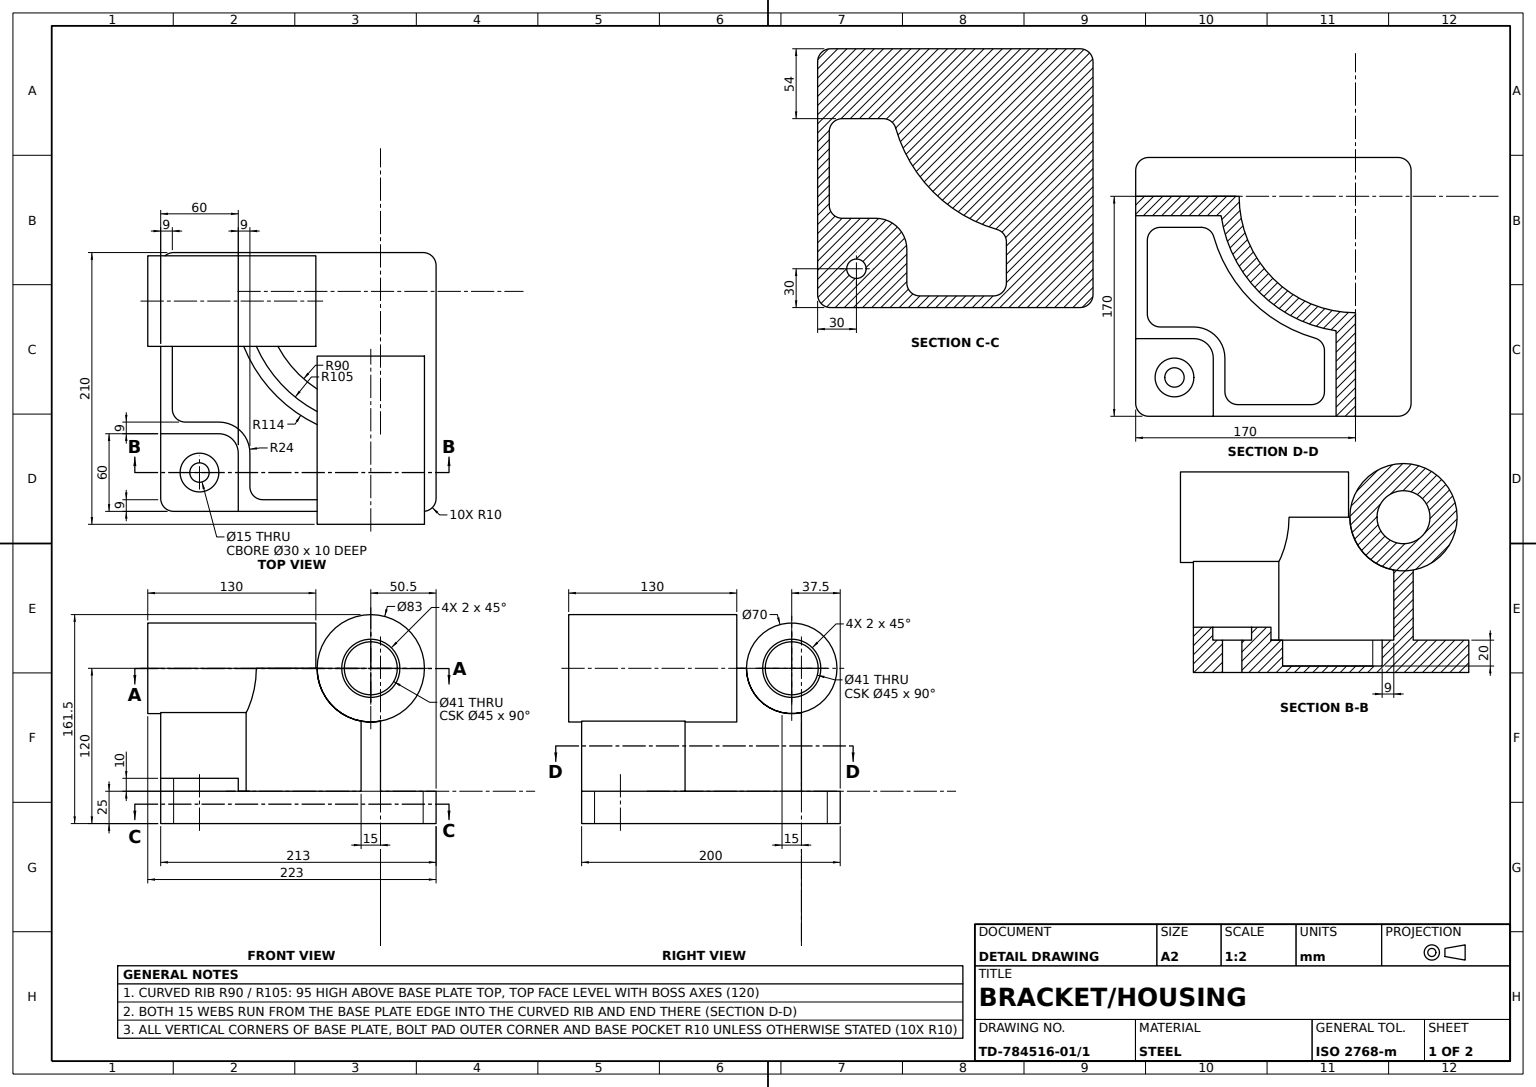
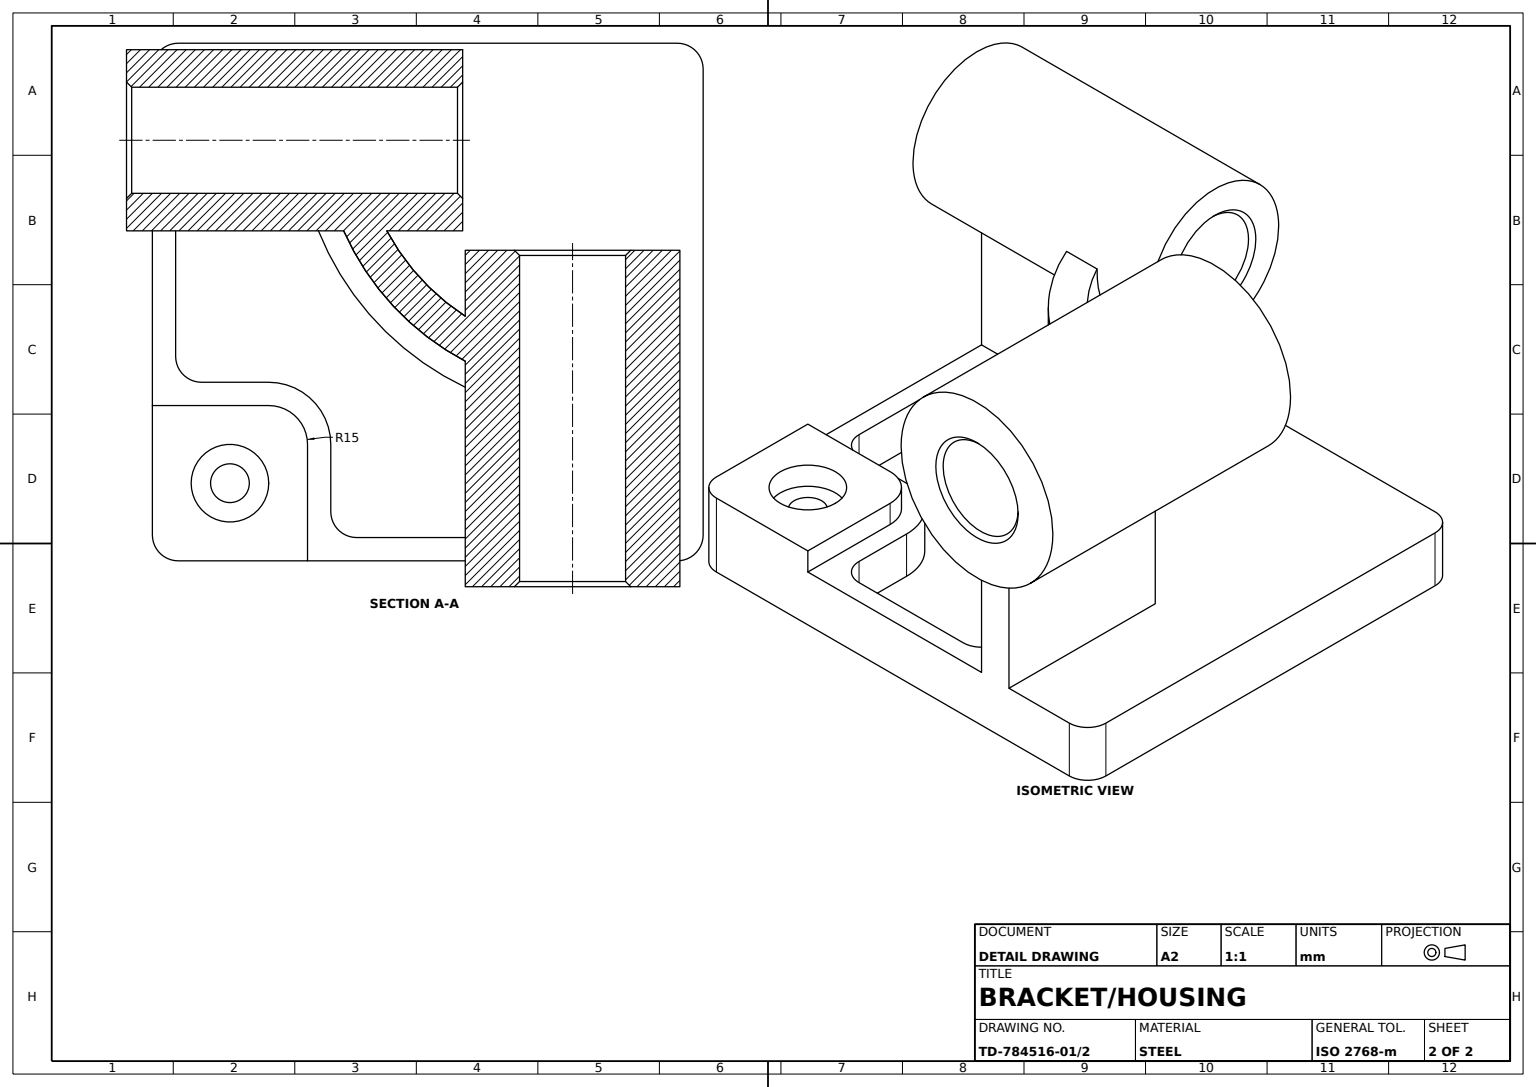
from build123d import *

# Parameters (mm, degrees)
BASE_PLATE_SKETCH_W                       = 200
BASE_PLATE_SKETCH_H                       = 213
BASE_PLATE_DEPTH                          = 25
BOLT_PAD_DEPTH                            = 10
BASE_PLATE_FILLETS_R10_R                  = 10
CENTRAL_HOUSING_DEPTH                     = 95
BEARING_BOSS_A_DEPTH                      = 10
BEARING_BOSS_A_DEPTH_BACK                 = 120
BEARING_BOSS_A_SKETCH_R                   = 35
BEARING_BOSS_B_DEPTH                      = 10
BEARING_BOSS_B_DEPTH_BACK                 = 120
BEARING_BOSS_B_SKETCH_R                   = 41.5
BEARING_BORE_A_41_REACH                   = 298.498
BEARING_BORE_A_SKETCH_R                   = 20.5
BEARING_BORE_B_41_REACH                   = 291.404
BEARING_BORE_B_SKETCH_R                   = 20.5
BORE_CHAMFERS_2X45_SIZE                   = 2
M8_COUNTERBORED_MOUNTING_HOLE_D           = 15
M8_COUNTERBORED_MOUNTING_HOLE_CBORE_D     = 30
M8_COUNTERBORED_MOUNTING_HOLE_CBORE_DEPTH = 10
BASE_POCKET_DEPTH                         = 20


with BuildPart() as part:
    # Base Plate Sketch → Base Plate (new body)
    with BuildSketch(Plane(origin=(0, 0, 0), x_dir=(1, 0, 0), z_dir=(0, 1, 0))):
        Rectangle(BASE_PLATE_SKETCH_W, BASE_PLATE_SKETCH_H)
    extrude(amount=BASE_PLATE_DEPTH)

    # Bolt Pad Sketch → Bolt Pad (add)
    with BuildSketch(Plane(origin=(0, 25, 0), x_dir=(1, 0, 0), z_dir=(0, 1, 0))):
        with BuildLine():
            Line((100, -106.5), (40, -106.5))
            Line((40, -106.5), (40, -61.5))
            ThreePointArc((40, -61.5), (44.393398282, -50.893398282), (55, -46.5))
            Line((55, -46.5), (100, -46.5))
            Line((100, -46.5), (100, -106.5))
        make_face()
    extrude(amount=BOLT_PAD_DEPTH)

    # Base Plate Fillets R10
    base_plate_fillets_r10_edges = [part.edges().sort_by_distance(p)[0] for p in [
        (100, 17.5, 106.5),
        (-100, 12.5, 106.5),
        (-100, 12.5, -106.5),
        (100, 12.5, -106.5),
    ]]
    fillet(base_plate_fillets_r10_edges, radius=BASE_PLATE_FILLETS_R10_R)

    # Central Housing Sketch → Central Housing (add)
    with BuildSketch(Plane(origin=(0, 25, 0), x_dir=(1, 0, 0), z_dir=(0, 1, 0))):
        with BuildLine():
            Line((100, 63.5), (20, 63.5))
            ThreePointArc((20, 63.5), (-6.360389693, -0.139610307), (-70, -26.5))
            Line((-70, -26.5), (-70, -106.5))
            Line((-70, -106.5), (-55, -106.5))
            Line((-55, -106.5), (-55, -40.423048454))
            ThreePointArc((-55, -40.423048454), (4.246212025, -10.746212025), (33.923048454, 48.5))
            Line((33.923048454, 48.5), (100, 48.5))
            Line((100, 48.5), (100, 63.5))
        make_face()
    extrude(amount=CENTRAL_HOUSING_DEPTH)

    # Bearing Boss A Sketch → Bearing Boss A (add, two sides: drawn at the far end of the back side and taken through both)
    with BuildSketch(Plane.XY.offset(106.5).offset(-BEARING_BOSS_A_DEPTH_BACK)):
        with Locations((-62.5, 120)):
            Circle(BEARING_BOSS_A_SKETCH_R)
    extrude(amount=BEARING_BOSS_A_DEPTH + BEARING_BOSS_A_DEPTH_BACK)

    # Bearing Boss B Sketch → Bearing Boss B (add, two sides: drawn at the far end of the back side and taken through both)
    with BuildSketch(Plane(origin=(100, 0, 0), x_dir=(0, 0, -1), z_dir=(1, 0, 0)).offset(-BEARING_BOSS_B_DEPTH_BACK)):
        with Locations((56, 120)):
            Circle(BEARING_BOSS_B_SKETCH_R)
    extrude(amount=BEARING_BOSS_B_DEPTH + BEARING_BOSS_B_DEPTH_BACK)

    # Bearing Bore A Sketch → Bearing Bore A Ø41 (cut, up to next)
    with BuildSketch(Plane.XY.offset(116.5), mode=Mode.PRIVATE) as bearing_bore_a_41_sk1:
        with Locations((-62.5, 120)):
            Circle(BEARING_BORE_A_SKETCH_R)
    bearing_bore_a_41_tool1 = extrude(bearing_bore_a_41_sk1.sketch, amount=-BEARING_BORE_A_41_REACH, mode=Mode.PRIVATE) & part.part
    add(bearing_bore_a_41_tool1.solids().sort_by_distance((-62.5, 120, 116.5))[0], mode=Mode.SUBTRACT)

    # Bearing Bore B Sketch → Bearing Bore B Ø41 (cut, up to next)
    with BuildSketch(Plane(origin=(110, 0, 0), x_dir=(0, 0, -1), z_dir=(1, 0, 0)), mode=Mode.PRIVATE) as bearing_bore_b_41_sk1:
        with Locations((56, 120)):
            Circle(BEARING_BORE_B_SKETCH_R)
    bearing_bore_b_41_tool1 = extrude(bearing_bore_b_41_sk1.sketch, amount=-BEARING_BORE_B_41_REACH, mode=Mode.PRIVATE) & part.part
    add(bearing_bore_b_41_tool1.solids().sort_by_distance((110, 120, -56))[0], mode=Mode.SUBTRACT)

    # Bore Chamfers 2x45°
    bore_chamfers_2x45_edges = [part.edges().sort_by_distance(p)[0] for p in [
        (-83, 120, 116.5),
        (-83, 120, -13.5),
        (110, 120, -35.5),
        (-20, 120, -35.5),
    ]]
    chamfer(bore_chamfers_2x45_edges, length=BORE_CHAMFERS_2X45_SIZE)

    # M8 Counterbored Mounting Hole (through all)
    with Locations(Plane(origin=(70, 35, 76.5), x_dir=(0, 0, 1), z_dir=(0, 1, 0))):
        with Locations((0, 0)):
            CounterBoreHole(M8_COUNTERBORED_MOUNTING_HOLE_D / 2, M8_COUNTERBORED_MOUNTING_HOLE_CBORE_D / 2, M8_COUNTERBORED_MOUNTING_HOLE_CBORE_DEPTH)

    # Base Pocket Sketch → Base Pocket (cut)
    with BuildSketch(Plane(origin=(0, 25, 0), x_dir=(1, 0, 0), z_dir=(0, 1, 0))):
        with BuildLine():
            Line((-46, -55.747641486), (-46, -87.5))
            ThreePointArc((-46, -87.5), (-43.071067812, -94.571067812), (-36, -97.5))
            Line((-36, -97.5), (21, -97.5))
            ThreePointArc((21, -97.5), (28.071067812, -94.571067812), (31, -87.5))
            Line((31, -87.5), (31, -61.5))
            ThreePointArc((31, -61.5), (38.029437252, -44.529437252), (55, -37.5))
            Line((55, -37.5), (81, -37.5))
            ThreePointArc((81, -37.5), (88.071067812, -34.571067812), (91, -27.5))
            Line((91, -27.5), (91, 29.5))
            ThreePointArc((91, 29.5), (88.071067812, 36.571067812), (81, 39.5))
            Line((81, 39.5), (49.247641486, 39.5))
            ThreePointArc((49.247641486, 39.5), (43.223496519, 37.481834214), (39.630896205, 32.241935484))
            ThreePointArc((39.630896205, 32.241935484), (10.610173055, -17.110173055), (-38.741935484, -46.130896205))
            ThreePointArc((-38.741935484, -46.130896205), (-43.981834214, -49.723496519), (-46, -55.747641486))
        make_face()
    extrude(amount=-BASE_POCKET_DEPTH, mode=Mode.SUBTRACT)


solid = part.part
